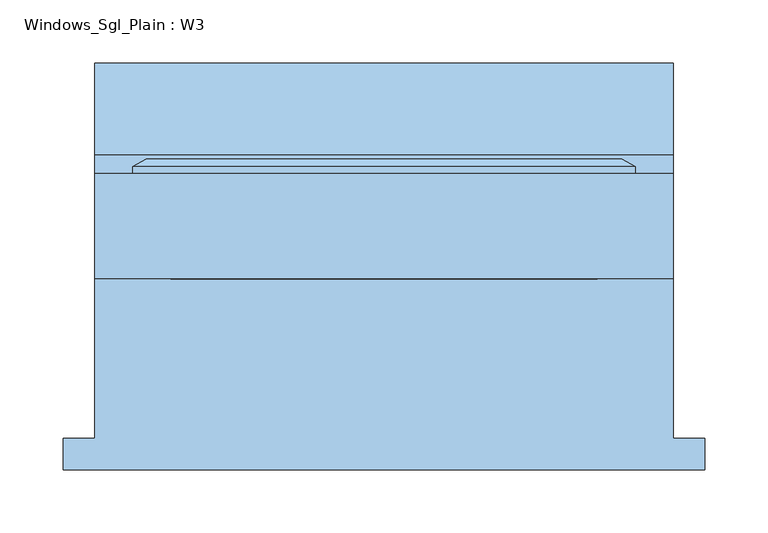
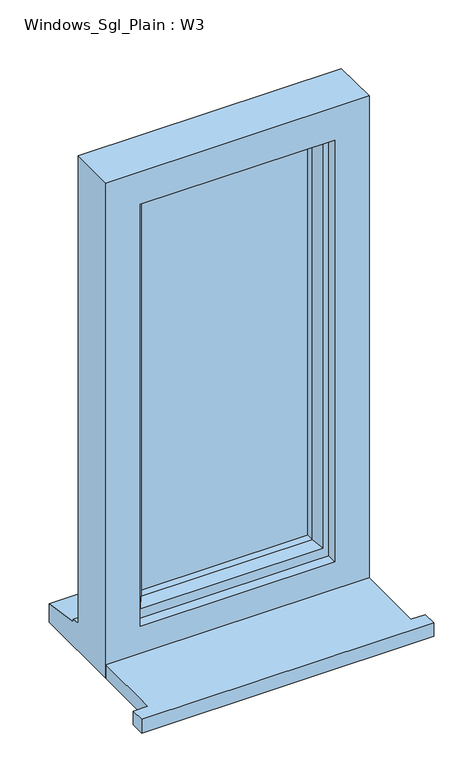
"""IFC4 building model written with IfcOpenShell, lengths in millimetres: window geometry, Windows_Sgl_Plain : W3."""

from ifc_helpers import new_model, si_unit, frame, origin, place, context, project, spatial, polyline, outline, extrude, faceted_brep, source, transform, mapped, element, save


def windows_sgl_plain_w3_7aa8ff83(model_context):
    return source(origin(), model_context, "Body", "SolidModel", [
        extrude(outline(polyline([(-253.6, -146.0834322), (-253.6, -121.0834322), (-228.6, -121.0834322), (-228.6, 4.9965678), (228.6, 4.9965678), (228.6, -121.0834322), (253.6, -121.0834322), (253.6, -146.0834322), (-253.6, -146.0834322)])), frame((0.0, 0.0, 1200.0), z_axis=(0.0, 0.0, 1.0), x_axis=(1.0, 0.0, 0.0)), (0.0, 0.0, 1.0), 25.0),
        faceted_brep([(-228.6, 4.9965678, 1200.0), (228.6, 4.9965678, 1200.0), (228.6, 4.9965678, 2110.0), (-228.6, 4.9965678, 2110.0), (-168.6, 4.9965678, 2050.0), (168.6, 4.9965678, 2050.0), (168.6, 4.9965678, 1275.0), (-168.6, 4.9965678, 1275.0), (-228.6, 87.9965678, 2110.0), (-228.6, 87.9965678, 1251.0), (-228.6, 102.9965678, 1249.68767), (-228.6, 102.9965678, 1244.7449676), (-228.6, 175.4965678, 1233.8088847), (-228.6, 175.4965678, 1200.0), (228.6, 87.9965678, 2110.0), (228.6, 87.9965678, 1251.0), (-188.6, 87.9965678, 2070.0), (-188.6, 87.9965678, 1263.0), (188.6, 87.9965678, 1263.0), (188.6, 87.9965678, 2070.0), (-188.6, 22.9965678, 2070.0), (-188.6, 22.9965678, 1263.0), (188.6, 22.9965678, 2070.0), (188.6, 22.9965678, 1263.0), (-168.6, 22.9965678, 2050.0), (-168.6, 22.9965678, 1275.0), (168.6, 22.9965678, 1275.0), (168.6, 22.9965678, 2050.0), (228.6, 175.4965678, 1200.0), (228.6, 175.4965678, 1233.8088847), (228.6, 102.9965678, 1244.7449676), (228.6, 102.9965678, 1249.68767)], [[[0, 1, 2, 3], [4, 5, 6, 7]], [[0, 3, 8, 9, 10, 11, 12, 13]], [[9, 8, 14, 15], [16, 17, 18, 19]], [[17, 16, 20, 21]], [[20, 22, 23, 21], [24, 25, 26, 27]], [[24, 4, 7, 25]], [[3, 2, 14, 8]], [[16, 19, 22, 20]], [[5, 4, 24, 27]], [[15, 14, 2, 1, 28, 29, 30, 31]], [[19, 18, 23, 22]], [[5, 27, 26, 6]], [[28, 1, 0, 13]], [[29, 28, 13, 12]], [[30, 29, 12, 11]], [[31, 30, 11, 10]], [[15, 31, 10, 9]], [[21, 23, 18, 17]], [[7, 6, 26, 25]]]),
        extrude(outline(polyline([(158.6, 51.9965678), (-158.6, 51.9965678), (-158.6, 75.9965678), (158.6, 75.9965678), (158.6, 51.9965678)])), frame((0.0, 0.0, 1293.0), z_axis=(0.0, 0.0, 1.0), x_axis=(1.0, 0.0, 0.0)), (0.0, 0.0, 1.0), 747.0),
        faceted_brep([(-198.6, 87.9965678, 2080.0), (-198.6, 93.7700705, 2080.0), (-198.6, 93.7700705, 1253.0), (-198.6, 87.9965678, 1253.0), (-188.6, 22.9965678, 2070.0), (-188.6, 87.9965678, 2070.0), (-188.6, 87.9965678, 1263.0), (-188.6, 22.9965678, 1263.0), (-148.6, 37.4894677, 2030.0), (-158.7480377, 22.9965678, 2040.1480377), (-158.7480377, 22.9965678, 1292.8519623), (-148.6, 37.4894677, 1303.0), (-148.6, 51.9965678, 2030.0), (-148.6, 51.9965678, 1303.0), (-158.6, 75.9965678, 2040.0), (-158.6, 51.9965678, 2040.0), (-158.6, 51.9965678, 1293.0), (-158.6, 75.9965678, 1293.0), (-148.6, 93.7700705, 2030.0), (-148.6, 75.9965678, 2030.0), (-148.6, 75.9965678, 1303.0), (-148.6, 93.7700705, 1303.0), (-166.0457548, 99.5435732, 2047.4457548), (-166.0457548, 99.5435732, 1285.5542452), (-187.8153903, 99.5435732, 2069.2153903), (-187.8153903, 99.5435732, 1263.7846097), (198.6, 93.7700705, 1253.0), (198.6, 87.9965678, 1253.0), (188.6, 87.9965678, 1263.0), (188.6, 22.9965678, 1263.0), (158.7480377, 22.9965678, 1292.8519623), (148.6, 37.4894677, 1303.0), (148.6, 51.9965678, 1303.0), (158.6, 51.9965678, 1293.0), (158.6, 75.9965678, 1293.0), (148.6, 75.9965678, 1303.0), (148.6, 93.7700705, 1303.0), (166.0457548, 99.5435732, 1285.5542452), (187.8153903, 99.5435732, 1263.7846097), (198.6, 93.7700705, 2080.0), (198.6, 87.9965678, 2080.0), (188.6, 87.9965678, 2070.0), (188.6, 22.9965678, 2070.0), (158.7480377, 22.9965678, 2040.1480377), (148.6, 37.4894677, 2030.0), (148.6, 51.9965678, 2030.0), (158.6, 51.9965678, 2040.0), (158.6, 75.9965678, 2040.0), (148.6, 75.9965678, 2030.0), (148.6, 93.7700705, 2030.0), (166.0457548, 99.5435732, 2047.4457548), (187.8153903, 99.5435732, 2069.2153903)], [[[0, 1, 2, 3]], [[4, 5, 6, 7]], [[8, 9, 10, 11]], [[12, 8, 11, 13]], [[14, 15, 16, 17]], [[18, 19, 20, 21]], [[22, 18, 21, 23]], [[1, 24, 25, 2]], [[3, 2, 26, 27]], [[7, 6, 28, 29]], [[11, 10, 30, 31]], [[13, 11, 31, 32]], [[17, 16, 33, 34]], [[21, 20, 35, 36]], [[23, 21, 36, 37]], [[2, 25, 38, 26]], [[27, 26, 39, 40]], [[29, 28, 41, 42]], [[31, 30, 43, 44]], [[32, 31, 44, 45]], [[34, 33, 46, 47]], [[36, 35, 48, 49]], [[37, 36, 49, 50]], [[26, 38, 51, 39]], [[40, 39, 1, 0]], [[3, 27, 40, 0], [5, 41, 28, 6]], [[42, 41, 5, 4]], [[7, 29, 42, 4], [9, 43, 30, 10]], [[44, 43, 9, 8]], [[45, 44, 8, 12]], [[15, 46, 33, 16], [13, 32, 45, 12]], [[47, 46, 15, 14]], [[17, 34, 47, 14], [19, 48, 35, 20]], [[49, 48, 19, 18]], [[50, 49, 18, 22]], [[24, 51, 38, 25], [23, 37, 50, 22]], [[39, 51, 24, 1]]]),
    ])


if __name__ == "__main__":
    model = new_model("IFC4")
    model_context = context("Model", 3, world=origin())
    ifc_project = project(units=[si_unit("LENGTHUNIT", "METRE", prefix="MILLI")], contexts=[model_context])
    site = spatial("IfcSite", under=ifc_project)
    building = spatial("IfcBuilding", under=site)
    placement = place(None, origin())
    windows_sgl_plain_w3_shape = windows_sgl_plain_w3_7aa8ff83(model_context)
    element("IfcWindow", 1, ObjectType="Windows_Sgl_Plain : W3", at=placement, inside=building, context=model_context, shape_type="MappedRepresentation", body=[
        mapped(windows_sgl_plain_w3_shape, transform((0.0, 0.0, 0.0), x_axis=(1.0, 0.0, 0.0), y_axis=(0.0, 1.0, 0.0), z_axis=(0.0, 0.0, 1.0))),
    ])
    save(model, "model.ifc")

# Revit data of these elements
# Type "Windows_Sgl_Plain : W3"
#   Type Mark = "58"
#   Operation = "SinglePanel"
#   Construction Type Id = "SGL"
#   Manufacturer = "Revit"
#   Keynote = "L10"
#   Analytic Construction = "Large single-glazed windows"
#   Wrap Layers (Ext) from Ext = 0.336286 ft
#   Wrap Layers (Int) from Ext = 0.582349 ft
#   Window Board Projection = 0.082021 ft
#   Window Board Extension = 0.082021 ft
#   Visual Light Transmittance = 0.9
#   Solar Heat Gain Coefficient = 0.86
#   Rough Width = 1.5 ft
#   Rough Height = 2.985564 ft
#   Height = 2.985564 ft
#   Width = 1.5 ft
#   Heat Transfer Coefficient (U) = 5.5617 W/(m²·K)
#   Glazing Thickness = 0.07874 ft
#   FrameOffset - External = 0.164042 ft
#   Frame Depth = 0.213255 ft
#   Default Head Height = 6.922572 ft
#   Cill Depth = 0.287073 ft
#   Cavity Closer Width = 0.164042 ft
#   Cavity Closer Offset from Ext = 0.336286 ft
#   Cavity Closer Depth = 0.278871 ft
#   Vis - Cavity Closers = yes
#   Define Thermal Properties by = 1
#   Material Trim = Window Frame
#   Material Glass = Glass
#   Material Frame = Window Frame
#   Wall Closure = (empty or 0)
# Element 1 (IfcWindow, "Windows_Sgl_Plain : W3")
#   Materials on its faces: "Window Frame", "Glass"
# Materials
#   "Window Frame": colour RGB 249 249 249, transparency 0, Keynote = "L10", Cost = 0
#   "Glass": class "Glass", colour RGB 0 128 192, transparency 0.9, Description = "Soda Lime Glass", Cost = 0
